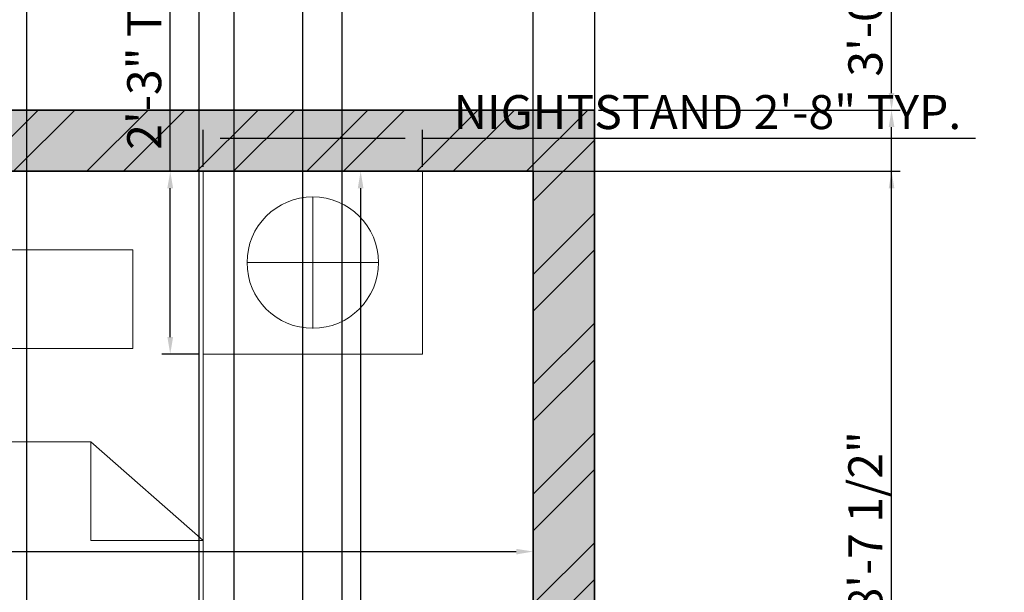
# Model space of a CAD drawing. Units: inches. Extents: x 1804 to 3296, y 909 to 2477.
# Tile 21 of 31: x 2241 to 2386, y 1722 to 1807. Entities that reach past the tile are written whole.
import ezdxf

# ---------------------------------------------------------------- set-up
doc = ezdxf.new("R2010")
doc.units = ezdxf.units.IN
for name, color, linetype, lineweight in [('A-ANNO-DIMS', 2, 'Continuous', 18), ('A-ANNO-TTLB', 156, 'Continuous', 35), ('A-WALL-PATT', 10, 'Continuous', 13), ('C-PROP', 7, 'Continuous', 25), ('FUR', 100, 'Continuous', 18), ('WALL', 10, 'Continuous', 35)]:
    doc.layers.add(name, color=color, linetype=linetype, lineweight=lineweight)
doc.styles.get("Standard").update_dxf_attribs({"font": 'arial.ttf'})
doc.dimstyles.new('ISO-25', dxfattribs={"dimtxt": 5, "dimasz": 2.5, "dimexe": 1.25, "dimexo": 0.625, "dimtad": 1, "dimdec": 0, "dimlunit": 4, "dimtxsty": 'Standard', "dimcen": 2.5, "dimadec": 0, "dimazin": 0, "dimtfac": 1, "dimtdec": 0, "dimtmove": 0, "dimatfit": 3, "dimfxl": 1, "dimarcsym": 0})

# ---------------------------------------------------------------- blocks, each defined once
blk = doc.blocks.new('*D10')
at = {"layer": 'A-ANNO-DIMS', "color": 0, "lineweight": -2, "transparency": 16777216}
for p, q in [((2119.08, 1783.75), (2119.08, 1727.15)), ((2316.54, 1783.75), (2316.54, 1727.15)), ((2121.58, 1728.4), (2314.04, 1728.4))]:
    blk.add_line(p, q, dxfattribs=at)
at = {"layer": 'A-ANNO-DIMS', "color": 0, "lineweight": 100, "transparency": 16777216}
for points in [[(2121.58, 1728.81), (2121.58, 1727.98), (2119.08, 1728.4)], [(2314.04, 1728.81), (2314.04, 1727.98), (2316.54, 1728.4)]]:
    blk.add_solid(points, dxfattribs=at)
at = {"layer": 'Defpoints', "color": 0, "lineweight": 100, "transparency": 16777216}
for p in [(2119.08, 1784.38), (2316.54, 1784.38), (2316.54, 1728.4)]:
    blk.add_point(p, dxfattribs=at)
at = {"layer": 'A-ANNO-DIMS', "color": 0, "transparency": 16777216, "insert": (2217.81, 1731.58), "char_height": 5, "attachment_point": 5}
blk.add_mtext('16\'-5"', dxfattribs=at)
blk = doc.blocks.new('*D11')
at = {"layer": 'A-ANNO-DIMS', "color": 0, "lineweight": -2, "transparency": 16777216}
for p, q in [((2315.91, 1784.38), (2289.92, 1784.38)), ((2291.17, 1781.88), (2291.17, 1593.42)), ((2315.91, 1590.92), (2289.92, 1590.92))]:
    blk.add_line(p, q, dxfattribs=at)
at = {"layer": 'A-ANNO-DIMS', "color": 0, "lineweight": 100, "transparency": 16777216}
for points in [[(2290.75, 1781.88), (2291.58, 1781.88), (2291.17, 1784.38)], [(2290.75, 1593.42), (2291.58, 1593.42), (2291.17, 1590.92)]]:
    blk.add_solid(points, dxfattribs=at)
at = {"layer": 'Defpoints', "color": 0, "lineweight": 100, "transparency": 16777216}
for p in [(2316.54, 1784.38), (2291.17, 1590.92), (2316.54, 1590.92)]:
    blk.add_point(p, dxfattribs=at)
at = {"layer": 'A-ANNO-DIMS', "color": 0, "transparency": 16777216, "insert": (2287.99, 1687.65), "char_height": 5, "attachment_point": 5, "rotation": 90}
blk.add_mtext('16\'-1"', dxfattribs=at)
blk = doc.blocks.new('NIGHTSTAND-WITH-LAMP')
for p, q in [((16.12, 3.78), (16.12, 23.13)), ((6.45, 13.46), (25.79, 13.46))]:
    blk.add_line(p, q)
blk.add_lwpolyline([(32.24, 26.91), (0, 26.91), (0, 0), (32.24, 0)], close=True)
blk.add_circle((16.12, 13.46), 9.67)
blk = doc.blocks.new('*D49')
at = {"layer": 'A-ANNO-DIMS', "color": 0, "lineweight": -2, "transparency": 16777216}
for p, q in [((2268, 1785), (2268, 1790.47)), ((2300.24, 1785), (2300.24, 1790.47)), ((2270.5, 1789.22), (2297.74, 1789.22)), ((2300.24, 1789.22), (2381.57, 1789.22))]:
    blk.add_line(p, q, dxfattribs=at)
at = {"layer": 'A-ANNO-DIMS', "color": 0, "lineweight": 100, "transparency": 16777216}
for points in [[(2270.5, 1789.63), (2270.5, 1788.8), (2268, 1789.22)], [(2297.74, 1789.63), (2297.74, 1788.8), (2300.24, 1789.22)]]:
    blk.add_solid(points, dxfattribs=at)
at = {"layer": 'Defpoints', "color": 0, "lineweight": 100, "transparency": 16777216}
for p in [(2300.24, 1789.22), (2268, 1784.38), (2300.24, 1784.38)]:
    blk.add_point(p, dxfattribs=at)
at = {"layer": 'A-ANNO-DIMS', "color": 0, "transparency": 16777216, "insert": (2342.16, 1792.43), "char_height": 5, "attachment_point": 5}
blk.add_mtext('NIGHTSTAND 2\'-8" TYP.', dxfattribs=at)
blk = doc.blocks.new('*D50')
at = {"layer": 'A-ANNO-DIMS', "color": 0, "lineweight": -2, "transparency": 16777216}
for p, q in [((2263.17, 1784.38), (2263.17, 1818.69)), ((2267.38, 1784.38), (2261.92, 1784.38)), ((2263.17, 1759.97), (2263.17, 1781.88)), ((2267.38, 1757.47), (2261.92, 1757.47))]:
    blk.add_line(p, q, dxfattribs=at)
at = {"layer": 'A-ANNO-DIMS', "color": 0, "lineweight": 100, "transparency": 16777216}
for points in [[(2262.75, 1781.88), (2263.59, 1781.88), (2263.17, 1784.38)], [(2262.75, 1759.97), (2263.59, 1759.97), (2263.17, 1757.47)]]:
    blk.add_solid(points, dxfattribs=at)
at = {"layer": 'Defpoints', "color": 0, "lineweight": 100, "transparency": 16777216}
for p in [(2263.17, 1784.38), (2268, 1784.38), (2268, 1757.47)]:
    blk.add_point(p, dxfattribs=at)
at = {"layer": 'A-ANNO-DIMS', "color": 0, "transparency": 16777216, "insert": (2259.99, 1802.79), "char_height": 5, "attachment_point": 5, "rotation": 90}
blk.add_mtext('2\'-3" TYP.', dxfattribs=at)
blk = doc.blocks.new('*D53')
at = {"layer": 'A-ANNO-DIMS', "color": 0, "lineweight": -2, "transparency": 16777216}
for p, q in [((2326.16, 1793.38), (2370.49, 1793.38)), ((2369.24, 1140.57), (2369.24, 1790.88)), ((2326.16, 1138.07), (2370.49, 1138.07))]:
    blk.add_line(p, q, dxfattribs=at)
at = {"layer": 'A-ANNO-DIMS', "color": 0, "lineweight": 100, "transparency": 16777216}
for points in [[(2368.82, 1790.88), (2369.65, 1790.88), (2369.24, 1793.38)], [(2368.82, 1140.57), (2369.65, 1140.57), (2369.24, 1138.07)]]:
    blk.add_solid(points, dxfattribs=at)
at = {"layer": 'Defpoints', "color": 0, "lineweight": 100, "transparency": 16777216}
for p in [(2325.54, 1793.38), (2369.24, 1793.38), (2325.54, 1138.07)]:
    blk.add_point(p, dxfattribs=at)
at = {"layer": 'A-ANNO-DIMS', "color": 0, "transparency": 16777216, "insert": (2366.03, 1465.72), "char_height": 5, "attachment_point": 5, "rotation": 90}
blk.add_mtext('54\'-7 1/2"', dxfattribs=at)
blk = doc.blocks.new('*D55')
at = {"layer": 'A-ANNO-DIMS', "color": 0, "lineweight": -2, "transparency": 16777216}
for p, q in [((2326.16, 1830.04), (2370.49, 1830.04)), ((2369.24, 1795.88), (2369.24, 1827.54)), ((2326.16, 1793.38), (2370.49, 1793.38))]:
    blk.add_line(p, q, dxfattribs=at)
at = {"layer": 'A-ANNO-DIMS', "color": 0, "lineweight": 100, "transparency": 16777216}
for points in [[(2368.82, 1827.54), (2369.65, 1827.54), (2369.24, 1830.04)], [(2368.82, 1795.88), (2369.65, 1795.88), (2369.24, 1793.38)]]:
    blk.add_solid(points, dxfattribs=at)
at = {"layer": 'Defpoints', "color": 0, "lineweight": 100, "transparency": 16777216}
for p in [(2325.54, 1830.04), (2369.24, 1830.04), (2325.54, 1793.38)]:
    blk.add_point(p, dxfattribs=at)
at = {"layer": 'A-ANNO-DIMS', "color": 0, "transparency": 16777216, "insert": (2366.03, 1811.71), "char_height": 5, "attachment_point": 5, "rotation": 90}
blk.add_mtext('3\'-0 1/2"', dxfattribs=at)
blk = doc.blocks.new('*D57')
at = {"layer": 'A-ANNO-DIMS', "color": 0, "lineweight": -2, "transparency": 16777216}
for p, q in [((2268.63, 1784.38), (2370.49, 1784.38)), ((2369.24, 1683.54), (2369.24, 1781.88)), ((2268.63, 1681.04), (2370.49, 1681.04))]:
    blk.add_line(p, q, dxfattribs=at)
at = {"layer": 'A-ANNO-DIMS', "color": 0, "lineweight": 100, "transparency": 16777216}
for points in [[(2368.82, 1781.88), (2369.65, 1781.88), (2369.24, 1784.38)], [(2368.82, 1683.54), (2369.65, 1683.54), (2369.24, 1681.04)]]:
    blk.add_solid(points, dxfattribs=at)
at = {"layer": 'Defpoints', "color": 0, "lineweight": 100, "transparency": 16777216}
for p in [(2268, 1784.38), (2369.24, 1784.38), (2268, 1681.04)]:
    blk.add_point(p, dxfattribs=at)
at = {"layer": 'A-ANNO-DIMS', "color": 0, "transparency": 16777216, "insert": (2366.03, 1732.71), "char_height": 5, "attachment_point": 5, "rotation": 90}
blk.add_mtext('8\'-7 1/2"', dxfattribs=at)
blk = doc.blocks.new('*D65')
at = {"layer": 'A-ANNO-DIMS', "color": 0, "lineweight": -2, "transparency": 16777216}
for p, q in [((2282.65, 1466.57), (2282.65, 1874.99)), ((2316.54, 1466.57), (2316.54, 1874.99)), ((2285.15, 1873.74), (2314.04, 1873.74))]:
    blk.add_line(p, q, dxfattribs=at)
at = {"layer": 'A-ANNO-DIMS', "color": 0, "lineweight": 100, "transparency": 16777216}
for points in [[(2285.15, 1874.15), (2285.15, 1873.32), (2282.65, 1873.74)], [(2314.04, 1874.15), (2314.04, 1873.32), (2316.54, 1873.74)]]:
    blk.add_solid(points, dxfattribs=at)
at = {"layer": 'Defpoints', "color": 0, "lineweight": 100, "transparency": 16777216}
for p in [(2316.54, 1873.74), (2282.65, 1465.94), (2316.54, 1465.94)]:
    blk.add_point(p, dxfattribs=at)
at = {"layer": 'A-ANNO-DIMS', "color": 0, "transparency": 16777216, "insert": (2299.6, 1876.91), "char_height": 5, "attachment_point": 5}
blk.add_mtext('2\'-10"', dxfattribs=at)
blk = doc.blocks.new('*D67')
at = {"layer": 'A-ANNO-DIMS', "color": 0, "lineweight": -2, "transparency": 16777216}
for p, q in [((2267.43, 1587.05), (2267.43, 1874.99)), ((2288.43, 1587.05), (2288.43, 1874.99)), ((2269.93, 1873.74), (2285.93, 1873.74))]:
    blk.add_line(p, q, dxfattribs=at)
at = {"layer": 'A-ANNO-DIMS', "color": 0, "lineweight": 100, "transparency": 16777216}
for points in [[(2269.93, 1874.15), (2269.93, 1873.32), (2267.43, 1873.74)], [(2285.93, 1874.15), (2285.93, 1873.32), (2288.43, 1873.74)]]:
    blk.add_solid(points, dxfattribs=at)
at = {"layer": 'Defpoints', "color": 0, "lineweight": 100, "transparency": 16777216}
for p in [(2288.43, 1873.74), (2267.43, 1586.42), (2288.43, 1586.42)]:
    blk.add_point(p, dxfattribs=at)
at = {"layer": 'A-ANNO-DIMS', "color": 0, "transparency": 16777216, "insert": (2277.93, 1876.91), "char_height": 5, "attachment_point": 5}
blk.add_mtext('1\'-9"', dxfattribs=at)
blk = doc.blocks.new('*D68')
at = {"layer": 'A-ANNO-DIMS', "color": 0, "lineweight": -2, "transparency": 16777216}
for p, q in [((2242.06, 1587.05), (2242.06, 1874.99)), ((2267.43, 1587.05), (2267.43, 1874.99)), ((2244.56, 1873.74), (2264.93, 1873.74)), ((2267.43, 1873.74), (2296.2, 1873.74))]:
    blk.add_line(p, q, dxfattribs=at)
at = {"layer": 'A-ANNO-DIMS', "color": 0, "lineweight": 100, "transparency": 16777216}
for points in [[(2244.56, 1874.15), (2244.56, 1873.32), (2242.06, 1873.74)], [(2264.93, 1874.15), (2264.93, 1873.32), (2267.43, 1873.74)]]:
    blk.add_solid(points, dxfattribs=at)
at = {"layer": 'Defpoints', "color": 0, "lineweight": 100, "transparency": 16777216}
for p in [(2267.43, 1873.74), (2242.06, 1586.42), (2267.43, 1586.42)]:
    blk.add_point(p, dxfattribs=at)
at = {"layer": 'A-ANNO-DIMS', "color": 0, "transparency": 16777216, "insert": (2283.07, 1876.95), "char_height": 5, "attachment_point": 5}
blk.add_mtext('2\'-1 1/2"', dxfattribs=at)
blk = doc.blocks.new('*D73')
at = {"layer": 'A-ANNO-DIMS', "color": 0, "lineweight": -2, "transparency": 16777216}
for p, q in [((2272.59, 1272.26), (2272.59, 1874.99)), ((2316.54, 1272.26), (2316.54, 1874.99)), ((2275.09, 1873.74), (2314.04, 1873.74))]:
    blk.add_line(p, q, dxfattribs=at)
at = {"layer": 'A-ANNO-DIMS', "color": 0, "lineweight": 100, "transparency": 16777216}
for points in [[(2275.09, 1874.15), (2275.09, 1873.32), (2272.59, 1873.74)], [(2314.04, 1874.15), (2314.04, 1873.32), (2316.54, 1873.74)]]:
    blk.add_solid(points, dxfattribs=at)
at = {"layer": 'Defpoints', "color": 0, "lineweight": 100, "transparency": 16777216}
for p in [(2316.54, 1873.74), (2272.59, 1271.63), (2316.54, 1271.63)]:
    blk.add_point(p, dxfattribs=at)
at = {"layer": 'A-ANNO-DIMS', "color": 0, "transparency": 16777216, "insert": (2294.56, 1876.92), "char_height": 5, "attachment_point": 5}
blk.add_mtext('3\'-8"', dxfattribs=at)

msp = doc.modelspace()

# ---------------------------------------------------------------- hatches: boundary and pattern name
at = {"layer": 'A-ANNO-TTLB'}
h = msp.add_hatch(color=256, dxfattribs=at)
h.dxf.hatch_style = 1
h.paths.add_polyline_path([(3294.53, 2476.54), (1803.79, 2476.54), (1805.43, 909.47), (3296.17, 909.47)])
h.paths.add_polyline_path([(1811, 914.33), (1812.79, 2467.54), (3285.53, 2467.54), (3283.74, 914.33)], flags=16)
h.paths.add_polyline_path([(1925.58, 1062.77), (1925.58, 1138.07), (1925.58, 1539.88), (1925.58, 1793.38), (1925.58, 1830.04), (2325.54, 1830.04), (2325.54, 1793.38), (2325.54, 1586.42), (2325.54, 1138.07), (2325.54, 1062.77)], flags=0)
h.paths.add_polyline_path([(1997.22, 1029.4), (2008.85, 1037.96), (2008.85, 1020.84)], flags=0)
h.paths.add_polyline_path([(1934.58, 1138.07), (1934.58, 1147.07), (2078.77, 1147.07), (2078.77, 1138.07), (2060.94, 1138.07)], flags=0)
h.paths.add_polyline_path([(1944.35, 1138.07), (1944.35, 1147.07), (2056.05, 1147.07), (2056.05, 1138.07)], flags=0)
h.paths.add_polyline_path([(2222.24, 1037.96), (2233.87, 1029.4), (2222.24, 1020.84)], flags=0)
h.paths.add_polyline_path([(2061.94, 1139.07), (2061.94, 1146.07), (2077.77, 1146.07), (2077.77, 1139.07)], flags=0)
h.paths.add_polyline_path([(2149.58, 1138.07), (2149.58, 1269.44), (2158.58, 1269.44), (2158.58, 1326.69), (2149.58, 1326.69), (2149.58, 1340.94), (2139.6, 1340.94), (2139.6, 1434.25), (2149.58, 1434.25), (2149.58, 1447.36), (2158.58, 1447.36), (2158.58, 1423.87), (2158.58, 1408.06), (2198.46, 1408.06), (2198.46, 1412.56), (2282.65, 1412.56), (2282.65, 1465.94), (2316.54, 1465.94), (2316.54, 1590.92), (2192.86, 1590.92), (2192.86, 1595.3), (2291.17, 1595.3), (2291.17, 1590.92), (2316.54, 1590.92), (2316.54, 1784.38), (2300.24, 1784.38), (2300.24, 1757.47), (2268, 1757.47), (2268, 1681.04), (2180.87, 1681.04), (2180.87, 1757.47), (2148.63, 1757.47), (2148.63, 1784.38), (2119.08, 1784.38), (2119.08, 1585.58), (2114.58, 1585.58), (2114.58, 1784.38), (2064.11, 1784.38), (2046.28, 1784.38), (2046.28, 1760.38), (1958.58, 1760.38), (1958.58, 1664.38), (1934.58, 1664.38), (1934.58, 1784.38), (1934.58, 1793.38), (2046.28, 1793.38), (2064.11, 1793.38), (2119.08, 1793.38), (2230.78, 1793.38), (2230.78, 1784.38), (2268, 1784.38), (2300.24, 1784.38), (2316.54, 1784.38), (2316.54, 1590.92), (2316.54, 1373.73), (2316.54, 1138.07)], flags=0)
h.paths.add_polyline_path([(2209.19, 1166.63), (2209.19, 1175.63), (2158.58, 1175.63), (2209.19, 1223.63), (2209.19, 1231.63), (2183.88, 1231.63), (2183.88, 1301.66), (2242.59, 1301.66), (2242.59, 1326.69), (2316.54, 1326.69), (2272.59, 1271.63), (2272.59, 1223.63), (2316.54, 1175.63), (2272.59, 1175.63), (2272.59, 1166.63)], flags=0)
h.paths.add_polyline_path([(1947.77, 1345.22), (1947.77, 1457.48), (1991.2, 1457.48), (1991.2, 1451.7), (1991.2, 1352.18), (1991.2, 1345.22)], flags=0)
h.paths.add_polyline_path([(2209.19, 1271.63), (2262.59, 1271.63), (2262.59, 1311.85), (2272.59, 1301.66), (2272.59, 1271.63), (2269.92, 1269.63), (2270.59, 1269.63), (2270.59, 1225.63), (2211.19, 1225.63), (2211.19, 1269.63), (2211.86, 1269.63)], flags=0)
h.paths.add_polyline_path([(2000.34, 1378.21), (2000.34, 1429.71), (2025.22, 1429.71), (2025.22, 1378.21)], flags=0)
h.paths.add_polyline_path([(2001.34, 1379.21), (2001.34, 1428.71), (2024.22, 1428.71), (2024.22, 1379.21)], flags=0)
h.paths.add_polyline_path([(2012.34, 1390.21), (2012.34, 1417.71), (2013.22, 1417.71), (2013.22, 1390.21)], flags=0)
h.paths.add_polyline_path([(2237.56, 1331.19), (2237.56, 1340.18), (2238.62, 1340.18), (2238.62, 1386.84), (2241.04, 1386.84), (2242.06, 1386.84), (2242.06, 1408.06), (2316.54, 1331.19)], flags=0)
h.paths.add_polyline_path([(1953.73, 1464.35), (1953.73, 1498.59), (1981.74, 1498.59), (1981.74, 1464.35)], flags=0)
h.paths.add_polyline_path([(1987.63, 1462.08), (1987.63, 1500.95), (2104.07, 1500.95), (2104.07, 1462.08), (2099.27, 1462.08), (1993.6, 1462.08)], flags=0)
h.paths.add_polyline_path([(1956.06, 1481.47, -1), (1979.41, 1481.47, -1)], flags=0)
edge = h.paths.add_edge_path(flags=0)
edge.add_ellipse((2299.53, 1438.37), major_axis=(0.31, 21.36), ratio=0.670333, start_angle=0, end_angle=360)
h.paths.add_polyline_path([(2297.39, 1438.37, -1), (2301.67, 1438.37, -1)], flags=0)
h.paths.add_polyline_path([(2591.54, 1163.23), (2591.54, 1179.38), (2591.54, 1379.68), (2591.54, 1395.84), (2734.5, 1395.84), (2734.5, 1379.68), (2734.5, 1179.38), (2734.5, 1163.23)], flags=0)
h.paths.add_polyline_path([(2592.54, 1164.23), (2592.54, 1166.23), (2733.5, 1166.23), (2733.5, 1164.23)], flags=0)
h.paths.add_polyline_path([(2592.54, 1180.38), (2592.54, 1378.68), (2733.5, 1378.68), (2733.5, 1180.38)], flags=0)
h.paths.add_polyline_path([(2593.54, 1181.38), (2593.54, 1377.68), (2732.5, 1377.68), (2732.5, 1181.38)], flags=0)
h.paths.add_polyline_path([(2594.54, 1182.38), (2594.54, 1376.68), (2731.5, 1376.68), (2731.5, 1182.38)], flags=0)
h.paths.add_polyline_path([(1936.95, 1697.46), (1936.95, 1736.46), (1955.41, 1736.46), (1955.41, 1697.46)], flags=0)
h.paths.add_polyline_path([(1938.48, 1718.36), (1938.48, 1734.92), (1953.65, 1734.92), (1953.65, 1718.36)], flags=0)
h.paths.add_polyline_path([(1944.75, 1726.64, -1), (1947.37, 1726.64, -1)], flags=0)
h.paths.add_polyline_path([(2592.54, 1394.84), (2733.5, 1394.84), (2733.5, 1392.84), (2592.54, 1392.84)], flags=0)
h.paths.add_polyline_path([(1976.61, 1762.5), (1976.61, 1781.44), (2012.79, 1781.44), (2012.79, 1762.5)], flags=0)
h.paths.add_polyline_path([(1979.57, 1771.97, -1), (1991.39, 1771.97, -1)], flags=0)
h.paths.add_polyline_path([(1995.36, 1771.97, -1), (2007.18, 1771.97, -1)], flags=0)
h.paths.add_polyline_path([(2251.51, 1744.53), (2268, 1730.05), (2251.51, 1730.05)], flags=0)
h.paths.add_polyline_path([(2047.28, 1785.38), (2047.28, 1792.38), (2063.11, 1792.38), (2063.11, 1785.38)], flags=0)
h.paths.add_polyline_path([(2155.08, 1770.92, -1), (2174.42, 1770.92, -1)], flags=0)
h.paths.add_polyline_path([(2188.59, 1758.27), (2188.59, 1772.81), (2222.3, 1772.81), (2222.3, 1758.27)], flags=0)
h.paths.add_polyline_path([(2223.97, 1758.27), (2223.97, 1772.81), (2257.68, 1772.81), (2257.68, 1758.27)], flags=0)
h.paths.add_polyline_path([(2274.45, 1770.92, -1), (2293.8, 1770.92, -1)], flags=0)
h.paths.add_polyline_path([(2591.54, 1582.09), (2591.54, 1782.39), (2734.5, 1782.39), (2734.5, 1582.09)], flags=0)
h.paths.add_polyline_path([(2592.54, 1583.09), (2592.54, 1781.39), (2733.5, 1781.39), (2733.5, 1583.09)], flags=0)
h.paths.add_polyline_path([(2593.54, 1584.09), (2593.54, 1780.39), (2732.5, 1780.39), (2732.5, 1584.09)], flags=0)
h.paths.add_polyline_path([(2594.54, 1585.09), (2594.54, 1779.39), (2731.5, 1779.39), (2731.5, 1585.09)], flags=0)
h.paths.add_polyline_path([(1922.17, 1978.79), (1922.17, 2295.08), (1922.17, 2296.08), (2115.67, 2296.08), (2115.67, 2384.31), (2115.67, 2385.31), (2322.12, 2385.31), (2323.12, 2385.31), (2323.12, 1979.79), (2323.12, 1978.79), (1923.17, 1978.79)], flags=0)
h.paths.add_polyline_path([(1922.17, 1978.79), (1922.17, 2051.31), (1922.17, 2214.86), (1922.17, 2296.08), (2115.67, 2296.08), (2115.67, 2385.31), (2323.12, 2385.31), (2323.12, 2280.42), (2323.12, 1978.79), (2115.67, 1978.79)], flags=0)
h.paths.add_polyline_path([(1923.17, 1979.79), (1923.17, 2050.31), (2115.67, 2050.31), (2115.67, 2051.31), (1923.17, 2051.31), (1923.17, 2213.86), (1923.17, 2214.86), (1923.17, 2295.08), (1990.02, 2295.08), (1990.02, 2214.86), (1991.02, 2214.86), (1991.02, 2295.08), (2115.67, 2295.08), (2115.67, 1979.79), (2116.67, 1979.79), (2116.67, 2304.18), (2116.67, 2384.31), (2322.12, 2384.31), (2322.12, 2280.42), (2322.12, 1979.79), (2115.67, 1979.79)], flags=0)
h.paths.add_polyline_path([(2972.46, 1192.5), (2972.46, 1196.92), (2995.47, 1196.92), (2995.47, 1255.47), (2995.09, 1255.47), (2987.42, 1249.39), (2980.08, 1255.47), (2978.05, 1255.47), (2978.05, 1257.24), (2995.47, 1257.24), (2995.47, 1261.58), (3015.37, 1261.58), (3015.37, 1333.28), (3015.37, 1414.4), (3032.82, 1414.4), (3032.82, 1333.28), (3032.82, 1261.58), (3052.66, 1261.58), (3052.66, 1255.47), (3079.86, 1255.47), (3078.72, 1254.57), (3081.47, 1252.29), (3078.56, 1249.99), (3075.81, 1252.26), (3072.57, 1249.69), (3070.36, 1251.52), (3067.67, 1249.39), (3060.34, 1255.47), (3052.66, 1255.47), (3052.66, 1196.92), (3054.58, 1196.92), (3074, 1196.92), (3074, 1192.5), (3052.66, 1192.5), (2995.47, 1192.5)], flags=0)
h.paths.add_polyline_path([(2490.75, 1979.27), (2490.75, 1980.27), (2596.87, 1980.27), (2596.87, 2051.8), (2596.87, 2052.8), (2596.87, 2216.35), (2596.87, 2297.57), (2717.32, 2297.57), (2710.57, 2305.62), (2724.07, 2305.62), (2717.32, 2297.57), (2782.37, 2297.57), (2782.37, 2395.8), (3006.82, 2395.8), (3006.82, 1981.27), (3093.73, 1981.27), (3093.73, 1980.27), (3047.51, 1980.27), (3046.37, 1979.37), (3049.11, 1977.1), (3046.2, 1974.79), (3043.46, 1977.07), (3040.21, 1974.49), (3038, 1976.32), (3035.32, 1974.2), (3027.98, 1980.27), (2871.83, 1980.27), (2871.83, 1981.27), (2791.37, 1981.27), (2791.37, 2050.8), (2597.87, 2050.8), (2597.87, 1980.27), (2597.87, 1979.27), (2546.27, 1979.27), (2545.12, 1978.37), (2547.87, 1976.1), (2544.96, 1973.79), (2542.22, 1976.07), (2538.97, 1973.49), (2536.76, 1975.32), (2534.07, 1973.2), (2526.74, 1979.27)], flags=0)
h.paths.add_polyline_path([(2597.87, 2051.8), (2606.87, 2051.8), (2606.87, 2258.39), (2597.87, 2258.39), (2597.87, 2296.57), (2606.87, 2296.57), (2606.87, 2262.39), (2782.37, 2262.39), (2782.37, 2296.57), (2790.37, 2296.57), (2790.37, 2262.39), (2791.37, 2262.39), (2791.37, 2305.67), (2791.37, 2385.8), (2996.82, 2385.8), (2996.82, 2339.85), (3006.82, 2339.85), (3006.82, 2250.12), (2997.82, 2250.12), (2997.82, 1981.27), (2996.82, 1981.27), (2872.83, 1981.27), (2872.83, 1991.8), (2871.83, 1991.8), (2871.83, 2050.8), (2790.37, 2050.8), (2597.87, 2050.8)], flags=0)
h.paths.add_polyline_path([(2179.93, 2153.92), (2179.93, 2353.97), (2259.98, 2353.97), (2259.98, 2153.92)], flags=0)
h.paths.add_polyline_path([(2180.93, 2154.92), (2180.93, 2352.97), (2258.98, 2352.97), (2258.98, 2154.92)], flags=0)
h.paths.add_polyline_path([(2960.87, 1608.49), (2960.87, 1753.62), (3070.9, 1753.62), (3070.9, 1608.49)], flags=0)
h.paths.add_polyline_path([(2961.87, 1609.49), (2961.87, 1752.62), (3069.9, 1752.62), (3069.9, 1609.49)], flags=0)
h.paths.add_polyline_path([(2962.87, 1610.49), (2962.87, 1751.62), (3068.9, 1751.62), (3068.9, 1610.49)], flags=0)
h.paths.add_polyline_path([(2963.87, 1611.49), (2963.87, 1750.62), (3067.9, 1750.62), (3067.9, 1611.49)], flags=0)
h.paths.add_polyline_path([(2782.37, 2051.8), (2782.37, 2216.32), (2791.37, 2216.32), (2791.37, 2051.8), (2872.83, 2051.8), (2872.83, 2068.56), (2884.67, 2068.56), (2884.67, 2085.33), (2896.51, 2085.33), (2896.51, 2102.09), (2908.36, 2102.09), (2908.36, 2118.85), (2920.2, 2118.85), (2920.2, 2135.62), (2932.05, 2135.62), (2932.05, 2145.3), (2925.08, 2145.3), (2925.08, 2203.2), (2996.82, 2203.2), (2996.82, 2145.3), (2953.82, 2145.3), (2872.83, 2051.8), (2790.37, 2051.8)], flags=0)
h.paths.add_polyline_path([(2717.32, 2238.65), (2710.57, 2246.7), (2724.07, 2246.7)], flags=0)
h.paths.add_polyline_path([(2003.09, 1122.79), (2017.16, 1122.79), (2017.16, 1138.74), (2003.09, 1138.74)], flags=8)
h.paths.add_polyline_path([(2174.76, 1792.72), (2188.83, 1792.72), (2188.83, 1808.66), (2174.76, 1808.66)], flags=8)
h.paths.add_polyline_path([(1987.95, 1792.51), (2002.02, 1792.51), (2002.02, 1808.45), (1987.95, 1808.45)], flags=8)
h.paths.add_polyline_path([(2148.79, 1289.26), (2160.46, 1289.26), (2160.46, 1305.2), (2148.79, 1305.2)], flags=8)
h.paths.add_polyline_path([(2115.36, 1133.57), (2127.04, 1133.57), (2127.04, 1149.51), (2115.36, 1149.51)], flags=8)
h.paths.add_polyline_path([(2237.58, 1421.48), (2249.25, 1421.48), (2249.25, 1437.43), (2237.58, 1437.43)], flags=8)
h.paths.add_polyline_path([(2134.99, 1584.32), (2146.66, 1584.32), (2146.66, 1600.26), (2134.99, 1600.26)], flags=8)
h.paths.add_polyline_path([(2101.95, 1557.31), (2113.62, 1557.31), (2113.62, 1573.25), (2101.95, 1573.25)], flags=8)
h.paths.add_polyline_path([(2937.85, 1156.77), (3120.41, 1156.77), (3120.41, 1185.72), (2937.85, 1185.72)], flags=8)
h.paths.add_polyline_path([(2980.71, 1786.71), (3050.06, 1786.71), (3050.06, 1802.66), (2980.71, 1802.66)], flags=8)
h.paths.add_polyline_path([(2869.28, 1661.96), (2938.62, 1661.96), (2938.62, 1690.8), (2869.28, 1690.8)], flags=8)
h.paths.add_polyline_path([(3092.27, 1674.86), (3161.62, 1674.86), (3161.62, 1690.8), (3092.27, 1690.8)], flags=8)
h.paths.add_polyline_path([(2980.71, 1674.86), (3050.06, 1674.86), (3050.06, 1690.8), (2980.71, 1690.8)], flags=8)
h.paths.add_polyline_path([(2649.07, 1678.23), (2674.53, 1678.23), (2674.53, 1714.76), (2649.07, 1714.76)], flags=8)
h.paths.add_polyline_path([(2530.84, 1981.63), (2549.13, 1981.63), (2549.13, 1997.57), (2530.84, 1997.57)], flags=8)
h.paths.add_polyline_path([(3031.29, 1981.77), (3049.58, 1981.77), (3049.58, 1997.71), (3031.29, 1997.71)], flags=8)
h.paths.add_polyline_path([(2715.38, 1911.9), (2851.54, 1911.9), (2851.54, 1940.85), (2715.38, 1940.85)], flags=8)
h.paths.add_polyline_path([(2015.23, 1927.36), (2205.42, 1927.36), (2205.42, 1956.3), (2015.23, 1956.3)], flags=8)
h.paths.add_polyline_path([(2671.84, 2057.84), (2702.75, 2057.84), (2702.75, 2073.79), (2671.84, 2073.79)], flags=8)
h.paths.add_polyline_path([(2678.5, 2316.52), (2765.26, 2316.52), (2765.26, 2332.46), (2678.5, 2332.46)], flags=8)
h.paths.add_polyline_path([(2678.48, 2271.96), (2736.41, 2271.96), (2736.41, 2287.9), (2678.48, 2287.9)], flags=8)
h.paths.add_polyline_path([(2019.2, 972.79), (2243.21, 972.79), (2243.21, 1001.74), (2019.2, 1001.74)], flags=8)
h.paths.add_polyline_path([(2097.06, 1021.56), (2132.16, 1021.56), (2132.16, 1037.51), (2097.06, 1037.51)], flags=8)
h.paths.add_polyline_path([(2182.47, 1360.48), (2207.35, 1360.48), (2207.35, 1376.42), (2182.47, 1376.42)], flags=8)
h.paths.add_polyline_path([(2261.12, 1361.77), (2295.01, 1361.77), (2295.01, 1377.71), (2261.12, 1377.71)], flags=8)
h.paths.add_polyline_path([(2245.75, 1511.51), (2278.44, 1511.51), (2278.44, 1527.46), (2245.75, 1527.46)], flags=8)
h.paths.add_polyline_path([(1991.16, 1296.29), (2060.51, 1296.29), (2060.51, 1312.23), (1991.16, 1312.23)], flags=8)
h.paths.add_polyline_path([(2187, 1651.35), (2246.71, 1651.35), (2246.71, 1667.29), (2187, 1667.29)], flags=8)
h.paths.add_polyline_path([(1976.49, 1684.81), (2068.63, 1684.81), (2068.63, 1700.76), (1976.49, 1700.76)], flags=8)
at = {"layer": 'A-WALL-PATT'}
h = msp.add_hatch(dxfattribs=at)
h.set_pattern_fill('ANSI32', color=256, scale=1.2)
h.set_pattern_definition([(45, (0, 196.207), (-8.08223, 8.08223), []), (45, (5.388, 196.207), (-8.08223, 8.08223), [])])
h.paths.add_polyline_path([(1934.58, 1784.38), (1934.58, 1793.38), (1925.58, 1793.38), (1925.58, 1539.88), (2119.08, 1539.88), (2119.08, 1545.58), (2114.58, 1545.58), (2114.58, 1544.38), (1934.58, 1544.38)])
h.paths.add_polyline_path([(2114.58, 1793.38), (2064.11, 1793.38), (2064.11, 1784.38), (2114.58, 1784.38)], flags=17)
h.paths.add_polyline_path([(2325.54, 1793.38), (2230.78, 1793.38), (2230.78, 1784.38), (2268, 1784.38), (2300.24, 1784.38), (2316.54, 1784.38), (2316.54, 1590.92), (2316.54, 1586.42), (2325.54, 1586.42)])
h.paths.add_polyline_path([(1944.35, 1147.07), (1934.58, 1147.07), (1934.58, 1138.07), (1944.35, 1138.07)])
h.paths.add_polyline_path([(2101.21, 1144.07, -0.01877), (2101.32, 1147.07), (2078.77, 1147.07), (2078.77, 1138.07), (2101.21, 1138.07)])
h.paths.add_polyline_path([(1934.58, 1539.88), (1925.58, 1539.88), (1925.58, 1138.07), (1934.58, 1138.07), (1934.58, 1147.07)])
h.paths.add_polyline_path([(2325.54, 1586.42), (2316.54, 1586.42), (2316.54, 1373.73), (2316.54, 1138.07), (2325.54, 1138.07), (2325.54, 1228.97)])
h.paths.add_polyline_path([(2158.58, 1423.87), (2158.58, 1447.36), (2149.58, 1447.36), (2149.58, 1423.87), (2149.58, 1340.94), (2149.58, 1326.69), (2158.58, 1326.69), (2158.58, 1354.23), (2158.58, 1402.2)])
h.paths.add_polyline_path([(2316.54, 1412.56), (2282.65, 1412.56), (2273.09, 1412.56), (2273.09, 1408.06), (2316.54, 1408.06)])
h.paths.add_polyline_path([(2273.09, 1412.56), (2242.06, 1412.56), (2242.06, 1408.06), (2273.09, 1408.06)])
h.paths.add_polyline_path([(2237.56, 1412.56), (2198.46, 1412.56), (2198.46, 1408.06), (2237.56, 1408.06)])
h.paths.add_polyline_path([(2242.06, 1408.06), (2237.56, 1408.06), (2237.56, 1386.84), (2242.06, 1386.84)])
h.paths.add_polyline_path([(2242.06, 1412.56), (2237.56, 1412.56), (2237.56, 1408.06), (2242.06, 1408.06)])
h.paths.add_polyline_path([(2158.58, 1269.44), (2149.58, 1269.44), (2149.58, 1138.07), (2158.58, 1138.07)])
h.paths.add_polyline_path([(2149.58, 1147.07), (2141.21, 1147.07), (2141.21, 1144.07), (2141.21, 1138.07), (2149.58, 1138.07)])
h.paths.add_polyline_path([(2272.59, 1175.63), (2209.19, 1175.63), (2209.19, 1166.63), (2272.59, 1166.63)])
h.paths.add_polyline_path([(2237.56, 1446.21), (2242.06, 1446.21), (2242.06, 1586.42), (2237.56, 1586.42)])
h.paths.add_polyline_path([(2242.06, 1414.58), (2237.56, 1414.58), (2237.56, 1412.56), (2242.06, 1412.56)])
h = msp.add_hatch(color=256, dxfattribs=at)
h.dxf.hatch_style = 1
h.paths.add_polyline_path([(2114.58, 1793.38), (2064.11, 1793.38), (2064.11, 1784.38), (2114.58, 1784.38)])
h.paths.add_polyline_path([(2119.08, 1793.38), (2114.58, 1793.38), (2114.58, 1585.58), (2119.08, 1585.58)])
h.paths.add_polyline_path([(2325.54, 1793.38), (2230.78, 1793.38), (2230.78, 1784.38), (2268, 1784.38), (2316.54, 1784.38), (2316.54, 1590.92), (2316.54, 1586.42), (2325.54, 1586.42)])
h.paths.add_polyline_path([(2316.54, 1331.19), (2158.58, 1331.19), (2158.58, 1326.69), (2316.54, 1326.69)])
h.paths.add_polyline_path([(2242.06, 1408.06), (2237.56, 1408.06), (2237.56, 1386.84), (2242.06, 1386.84)])
h.paths.add_polyline_path([(2242.06, 1412.56), (2237.56, 1412.56), (2237.56, 1408.06), (2242.06, 1408.06)])
h.paths.add_polyline_path([(2237.56, 1412.56), (2198.46, 1412.56), (2198.46, 1408.06), (2237.56, 1408.06)])
h.paths.add_polyline_path([(2273.09, 1412.56), (2242.06, 1412.56), (2242.06, 1408.06), (2273.09, 1408.06)])
h.paths.add_polyline_path([(2316.54, 1412.56), (2282.65, 1412.56), (2273.09, 1412.56), (2273.09, 1408.06), (2316.54, 1408.06)])
h.paths.add_polyline_path([(2325.54, 1586.42), (2316.54, 1586.42), (2316.54, 1373.73), (2316.54, 1138.07), (2325.54, 1138.07), (2325.54, 1228.97)])
h.paths.add_polyline_path([(2272.59, 1175.63), (2209.19, 1175.63), (2209.19, 1166.63), (2272.59, 1166.63)])

# ---------------------------------------------------------------- linework, layer by layer
at = {"layer": 'C-PROP'}
msp.add_line((2325.54, 1830.04), (2325.54, 1793.38), dxfattribs=at)
at = {"layer": 'FUR'}
for p, q in [((2180.87, 1744.53), (2251.51, 1744.53)), ((2251.51, 1744.53), (2251.51, 1730.05)), ((2268, 1730.05), (2251.51, 1744.53)), ((2251.51, 1730.05), (2268, 1730.05))]:
    msp.add_line(p, q, dxfattribs=at)
for points in [[(2180.87, 1784.38), (2268, 1784.38), (2268, 1681.04), (2180.87, 1681.04)], [(2223.97, 1772.81), (2257.68, 1772.81), (2257.68, 1758.27), (2223.97, 1758.27)]]:
    msp.add_lwpolyline(points, close=True, dxfattribs=at)
at = {"layer": 'WALL'}
for p, q in [((2119.08, 1793.38), (2325.54, 1793.38)), ((2325.54, 1793.38), (2325.54, 1586.42)), ((2119.08, 1784.38), (2316.54, 1784.38)), ((2316.54, 1784.38), (2316.54, 1590.92))]:
    msp.add_line(p, q, dxfattribs=at)

# ---------------------------------------------------------------- block references
at = {"layer": 'FUR'}
msp.add_blockref('NIGHTSTAND-WITH-LAMP', (2268.01, 1757.47), dxfattribs=at)

# ---------------------------------------------------------------- dimensions: what is measured, and where the dimension line sits
at = {"layer": 'A-ANNO-DIMS'}
for base, p1, p2, override, picture, middle in [((2267.43, 1873.74), (2242.06, 1586.42), (2267.43, 1586.42), {"dimdec": 1, "dimlfac": 1, "dimrnd": 0, "dimzin": 1, "dimdsep": 46, "dimlunit": 4, "dimfrac": 2}, '*D68', (2283.07, 1876.95)), ((2288.43, 1873.74), (2267.43, 1586.42), (2288.43, 1586.42), {"dimdec": 1, "dimlfac": 1, "dimrnd": 0, "dimzin": 1, "dimdsep": 46, "dimlunit": 4, "dimfrac": 2}, '*D67', (2277.93, 1876.91)), ((2316.5375, 1873.7362), (2272.5886, 1271.6342), (2316.5375, 1271.6342), {"dimdec": 1, "dimlfac": 1, "dimrnd": 0, "dimzin": 1, "dimdsep": 46, "dimlunit": 4, "dimfrac": 2}, '*D73', (2294.563, 1876.9158)), ((2316.54, 1873.74), (2282.65, 1465.94), (2316.54, 1465.94), {"dimdec": 1, "dimlfac": 1, "dimrnd": 0, "dimzin": 1, "dimdsep": 46, "dimlunit": 4, "dimfrac": 2}, '*D65', (2299.6, 1876.91)), ((2316.54, 1728.4), (2119.08, 1784.38), (2316.54, 1784.38), {"dimclrd": 0, "dimclre": 0, "dimclrt": 0}, '*D10', (2217.81, 1731.58))]:
    dim = msp.add_linear_dim(base=base, p1=p1, p2=p2, dimstyle='ISO-25', override=override, dxfattribs=at)
    dim.commit()
    dim.dimension.update_dxf_attribs({"geometry": picture, "text_midpoint": middle})
for base, p1, p2, override, picture, middle in [((2369.24, 1830.04), (2325.54, 1793.38), (2325.54, 1830.04), {"dimdec": 1, "dimlfac": 1, "dimrnd": 0, "dimzin": 1, "dimdsep": 46, "dimlunit": 4, "dimfrac": 2}, '*D55', (2366.03, 1811.71)), ((2369.24, 1793.38), (2325.54, 1138.07), (2325.54, 1793.38), {"dimdec": 1, "dimlfac": 1, "dimrnd": 0, "dimzin": 1, "dimdsep": 46, "dimlunit": 4, "dimfrac": 2}, '*D53', (2366.03, 1465.72)), ((2369.24, 1784.38), (2268, 1681.04), (2268, 1784.38), {"dimdec": 1, "dimlfac": 1, "dimrnd": 0, "dimzin": 1, "dimdsep": 46, "dimlunit": 4, "dimfrac": 2}, '*D57', (2366.03, 1732.71)), ((2291.17, 1590.92), (2316.54, 1784.38), (2316.54, 1590.92), {"dimclrd": 0, "dimclre": 0, "dimclrt": 0}, '*D11', (2287.99, 1687.65))]:
    dim = msp.add_linear_dim(base=base, p1=p1, p2=p2, angle=90, dimstyle='ISO-25', override=override, dxfattribs=at)
    dim.commit()
    dim.dimension.update_dxf_attribs({"geometry": picture, "text_midpoint": middle})
dim = msp.add_linear_dim(base=(2263.17, 1784.38), p1=(2268, 1757.47), p2=(2268, 1784.38), angle=90, text='<> TYP.', dimstyle='ISO-25', override={"dimdec": 1, "dimlfac": 1, "dimrnd": 0, "dimzin": 1, "dimdsep": 46, "dimlunit": 4, "dimfrac": 2}, dxfattribs=at)
dim.commit()
dim.dimension.update_dxf_attribs({"geometry": '*D50', "text_midpoint": (2259.99, 1802.79)})
dim = msp.add_linear_dim(base=(2300.24, 1789.22), p1=(2268, 1784.38), p2=(2300.24, 1784.38), text='NIGHTSTAND <> TYP.', dimstyle='ISO-25', override={"dimdec": 1, "dimlfac": 1, "dimrnd": 0, "dimzin": 1, "dimdsep": 46, "dimlunit": 4, "dimfrac": 2}, dxfattribs=at)
dim.commit()
dim.dimension.update_dxf_attribs({"geometry": '*D49', "text_midpoint": (2342.16, 1792.43)})

doc.saveas('drawing.dxf')
